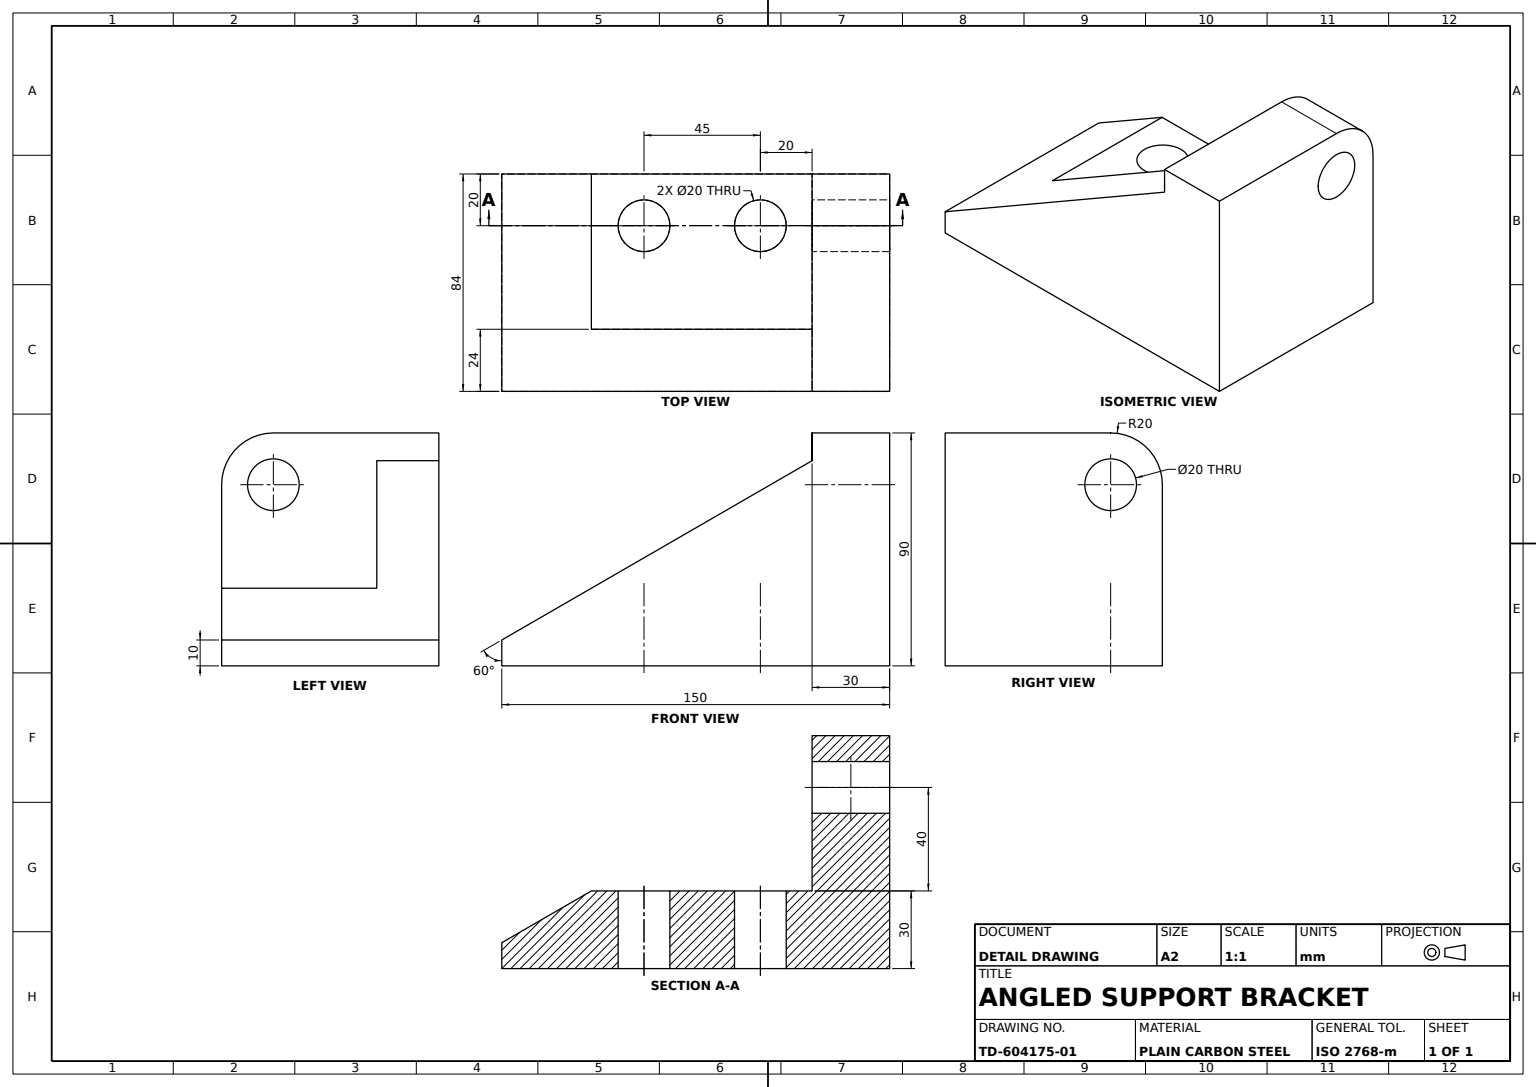
SolidWorks part; units mm, degrees
material "Plain Carbon Steel"
ref_plane "Front Plane" through (0, 0, 0) normal (0, 0, 1) x (1, 0, 0)
ref_plane "Top Plane" through (0, 0, 0) normal (0, 1, 0) x (1, 0, 0)
ref_plane "Right Plane" through (0, 0, 0) normal (1, 0, 0) x (0, 0, -1)
sketch "Bracket Profile Sketch" plane through (0, 0, 0) normal (1, 0, 0) x (0, 0, -1)
  line L0 (0, 0) -> (150, 0)
  line L1 (150, 0) -> (150, 90)
  line L2 (0, 0) -> (0, 10)
  line L3 (150, 90) -> (120, 90)
  line L4 (120, 90) -> (120, 70)
  line L5 (120, 79.282) -> (0, 10)
  line L6 (120, 70) -> (120, 30)
  line L7 (120, 30) -> (34.641, 30)
  line L8 (0, 10) -> (0, 47.0676)
  dimension "D1" = 10
  dimension "D2" = 90
  dimension "D3" = 150
  dimension "D4" = 30
  dimension "D5" = 20
  dimension "D6" = 40
  dimension "D7" = 60
  dimension "D8" = 47.0676
extrude "Bracket Body" add sketch "Bracket Profile Sketch" against normal blind 84 contours L6 L7 L5 L2 L0 L1 L3 L4
sketch "Gusset Sketch" plane through (0, 0, 0) normal (1, 0, 0) x (0, 0, -1)
  line L0 (34.641, 30) -> (120, 79.282)
  line L1 (120, 90) -> (120, 30) construction
  line L2 (120, 79.282) -> (120, 30)
  line L3 (120, 30) -> (34.641, 30)
  dimension "D1" = 49.282
extrude "Gusset" add sketch "Gusset Sketch" against normal blind 24
sketch "Base Holes Sketch" plane through (0, 0, 0) normal (0, 1, 0) x (1, 0, 0)
  line L0 (-84, 120) -> (0, 120) construction
  line L1 (-84, 120) -> (-84, 34.641) construction
  circle A0 centre (-64, 100) radius 10
  circle A1 centre (-64, 55) radius 10
  dimension "D5" = 20
  dimension "D6" = 20
  dimension "D1" = 20
  dimension "D2" = 20
  dimension "D3" = 45
  dimension "D4" = 20
extrude "Base Holes 2xØ20" cut sketch "Base Holes Sketch" along normal blind 30
sketch "Lug Hole Sketch" plane through (0, 0, 0) normal (0, 0, 1) x (1, 0, 0)
  line L0 (-84, 90) -> (-84, 30) construction
  line L1 (-84, 90) -> (0, 90) construction
  circle A0 centre (-64, 70) radius 10
  dimension "D3" = 20
  dimension "D1" = 20
  dimension "D2" = 20
extrude "Lug Hole Ø20" cut sketch "Lug Hole Sketch" against normal blind 208
fillet "Lug Top Fillet R20" radius 20 1 edges at (-84, 90, -135)
